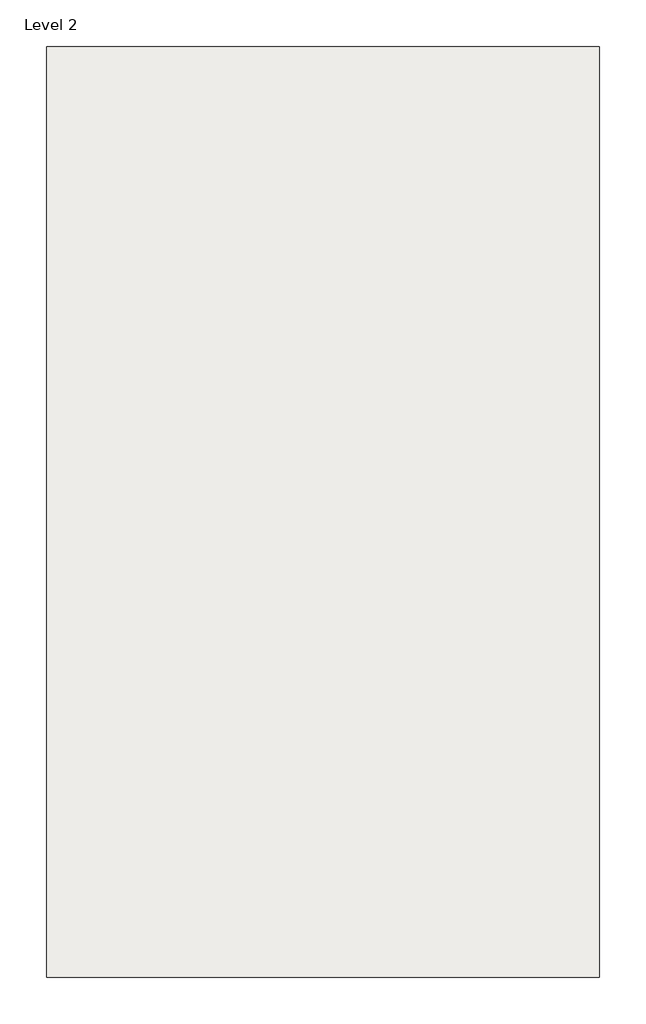
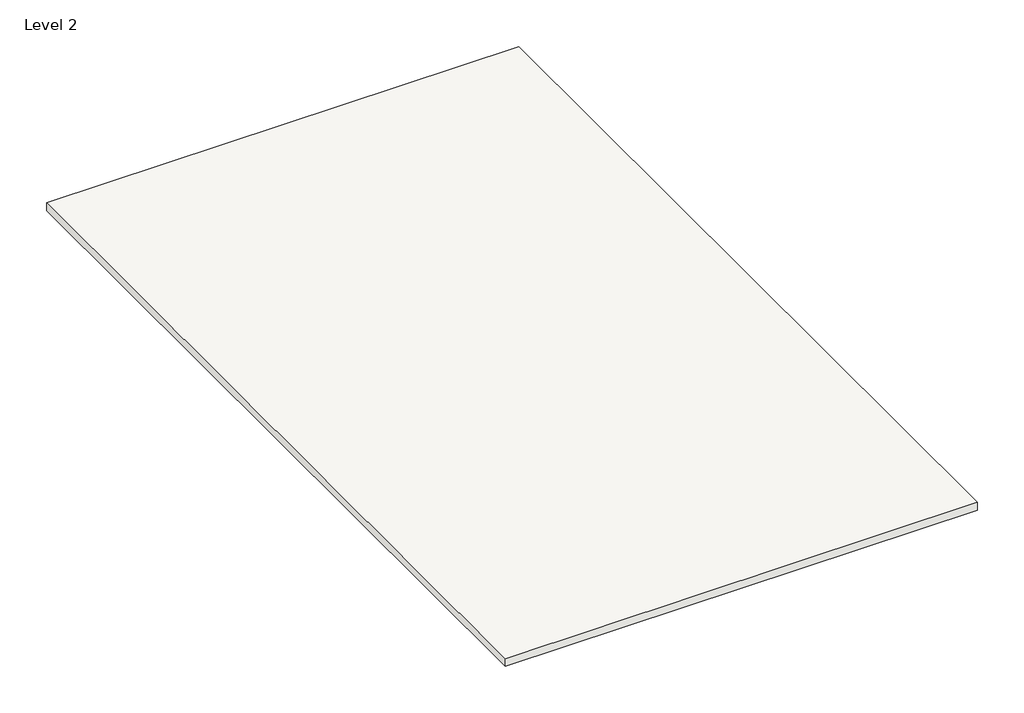
# One storey, incomplete: 1 roof.
"""IFC4 building model written with IfcOpenShell, lengths in millimetres."""

from ifc_helpers import new_model, si_unit, frame, origin, place, context, project, spatial, polyline, outline, extrude, element, save

model = new_model("IFC4")

# Units and contexts
model_context = context("Model", 3, world=origin())
ifc_project = project(units=[si_unit("LENGTHUNIT", "METRE", prefix="MILLI")], contexts=[model_context])

# Site, building, storey
site = spatial("IfcSite", under=ifc_project)
building = spatial("IfcBuilding", under=site)
storey = spatial("IfcBuildingStorey", under=building, Name="Level 2", Elevation=3048.0)

# Roof
placement = place(None, origin())
element("IfcRoof", 1, ObjectType="Generic - 12\"", at=placement, inside=storey, context=model_context, shape_type="SweptSolid", body=[
    extrude(outline(polyline([(-5674.8415084, 8005.7935985), (3164.3584916, 8005.7935985), (3164.3584916, -6872.2564015), (-5674.8415084, -6872.2564015), (-5674.8415084, 8005.7935985)])), frame((0.0, 0.0, 3048.0), z_axis=(0.0, 0.0, 1.0), x_axis=(1.0, 0.0, 0.0)), (0.0, 0.0, 1.0), 152.4),
])

save(model, "model.ifc")

# Revit data of these elements
# Type "Generic - 12\""
#   Assembly Code = "B1020"
#   Layers, outside or top first: 0' - 6" no material (function 1)
# Element 1 (IfcRoof, "Generic - 12\"")
#   built-in parameter 1001705 = 10.5 (stored number, unit not read)
#   built-in parameter 1001710 = 33615
#   Phase Created = New Construction
#   Materials on its faces: "Default Roof"
# Materials
#   "Default Roof": colour RGB 88 101 114, transparency 0, Cost = 0
